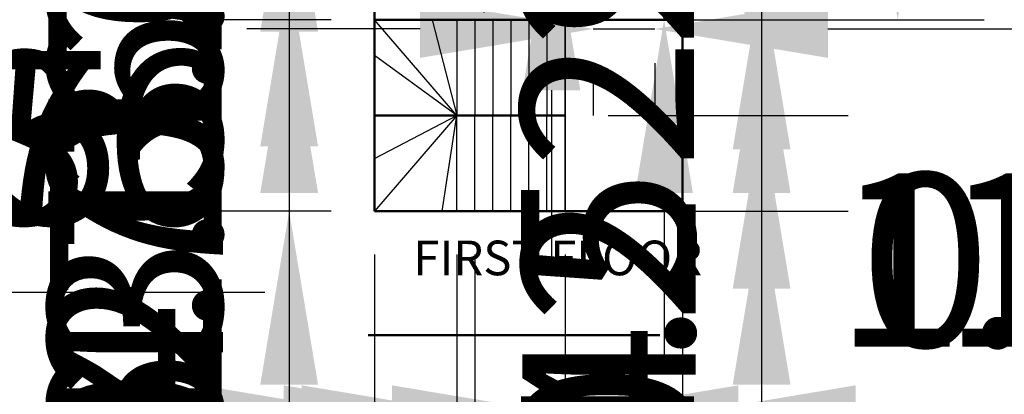
# Model space of a CAD drawing. Units: metres. Extents: x 782 to 1487, y 1262 to 7446.
# Tile 5 of 25: x 807.01 to 821.23, y 1287.66 to 1293.07. Entities that reach past the tile are written whole.
import ezdxf

# ---------------------------------------------------------------- set-up
doc = ezdxf.new("R2010")
doc.units = ezdxf.units.M
for name, color, linetype, lineweight in [('A-ANNO-DIMS', 2, 'Continuous', 18), ('A-ANNO-TEXT', 3, 'Continuous', 18), ('A-FLOR-STRS', 3, 'Continuous', 25), ('A-WALL', 7, 'Continuous', 50)]:
    doc.layers.add(name, color=color, linetype=linetype, lineweight=lineweight)
doc.styles.get("Standard").update_dxf_attribs({"font": 'arial.ttf'})
doc.dimstyles.new('ISO-25', dxfattribs={"dimtxt": 2.5, "dimasz": 2.5, "dimexe": 1.25, "dimexo": 0.625, "dimtad": 1, "dimtxsty": 'Standard', "dimcen": 2.5, "dimadec": 0, "dimazin": 0, "dimtfac": 1, "dimtmove": 0, "dimatfit": 3, "dimfxl": 1, "dimarcsym": 0})

# ---------------------------------------------------------------- blocks, each defined once
blk = doc.blocks.new('*D4')
at = {"layer": 'A-ANNO-DIMS', "color": 0, "lineweight": -2, "transparency": 16777216}
for p, q in [((817.205, 1307.327), (820.936, 1307.327)), ((819.686, 1304.827), (819.686, 1295.567)), ((817.205, 1293.067), (820.936, 1293.067))]:
    blk.add_line(p, q, dxfattribs=at)
at = {"layer": 'A-ANNO-DIMS', "color": 0, "transparency": 16777216}
for points in [[(819.269, 1304.827), (820.103, 1304.827), (819.686, 1307.327)], [(819.269, 1295.567), (820.103, 1295.567), (819.686, 1293.067)]]:
    blk.add_solid(points, dxfattribs=at)
at = {"layer": 'Defpoints', "color": 0, "transparency": 16777216}
for p in [(816.58, 1307.327), (816.58, 1293.067), (819.686, 1293.067)]:
    blk.add_point(p, dxfattribs=at)
at = {"layer": 'A-ANNO-DIMS', "color": 0, "transparency": 16777216, "insert": (817.558, 1300.197), "char_height": 2.5, "attachment_point": 5, "rotation": 90}
blk.add_mtext('14,26', dxfattribs=at)
blk = doc.blocks.new('*D22')
at = {"layer": 'A-ANNO-DIMS', "color": 0, "lineweight": -2, "transparency": 16777216}
for p, q in [((812.79, 1292.934), (810.29, 1292.934)), ((815.29, 1292.934), (816.179, 1292.934)), ((818.679, 1292.934), (848.834, 1292.934)), ((815.29, 1292.442), (815.29, 1291.684)), ((816.179, 1292.442), (816.179, 1291.684))]:
    blk.add_line(p, q, dxfattribs=at)
at = {"layer": 'A-ANNO-DIMS', "color": 0, "transparency": 16777216}
for points in [[(812.79, 1293.351), (812.79, 1292.517), (815.29, 1292.934)], [(818.679, 1293.351), (818.679, 1292.517), (816.179, 1292.934)]]:
    blk.add_solid(points, dxfattribs=at)
at = {"layer": 'Defpoints', "color": 0, "transparency": 16777216}
for p in [(815.29, 1293.067), (816.179, 1293.067), (816.179, 1292.934)]:
    blk.add_point(p, dxfattribs=at)
at = {"layer": 'A-ANNO-DIMS', "color": 0, "transparency": 16777216, "insert": (835.007, 1294.852), "char_height": 2.5, "attachment_point": 5}
blk.add_mtext('DOOR 0.89 TYP.', dxfattribs=at)
blk = doc.blocks.new('*D23')
at = {"layer": 'A-ANNO-DIMS', "color": 0, "lineweight": -2, "transparency": 16777216}
for p, q in [((816.313, 1296.414), (816.313, 1315.246)), ((816.313, 1293.067), (816.313, 1293.914)), ((816.804, 1293.914), (817.563, 1293.914)), ((816.804, 1293.067), (817.563, 1293.067)), ((816.313, 1290.567), (816.313, 1288.067))]:
    blk.add_line(p, q, dxfattribs=at)
at = {"layer": 'A-ANNO-DIMS', "color": 0, "transparency": 16777216}
for points in [[(815.896, 1296.414), (816.729, 1296.414), (816.313, 1293.914)], [(815.896, 1290.567), (816.729, 1290.567), (816.313, 1293.067)]]:
    blk.add_solid(points, dxfattribs=at)
at = {"layer": 'Defpoints', "color": 0, "transparency": 16777216}
for p in [(816.179, 1293.914), (816.313, 1293.914), (816.179, 1293.067)]:
    blk.add_point(p, dxfattribs=at)
at = {"layer": 'A-ANNO-DIMS', "color": 0, "transparency": 16777216, "insert": (814.411, 1307.08), "char_height": 2.5, "attachment_point": 5, "rotation": 90}
blk.add_mtext('0.85 TYP.', dxfattribs=at)
blk = doc.blocks.new('*D24')
at = {"layer": 'A-ANNO-DIMS', "color": 0, "lineweight": -2, "transparency": 16777216}
for p, q in [((811.209, 1294.423), (808.709, 1294.423)), ((813.709, 1294.423), (814.559, 1294.423)), ((817.059, 1294.423), (852.649, 1294.423)), ((813.709, 1293.926), (813.709, 1293.173)), ((814.559, 1293.926), (814.559, 1293.173))]:
    blk.add_line(p, q, dxfattribs=at)
at = {"layer": 'A-ANNO-DIMS', "color": 0, "transparency": 16777216}
for points in [[(811.209, 1294.84), (811.209, 1294.006), (813.709, 1294.423)], [(817.059, 1294.84), (817.059, 1294.006), (814.559, 1294.423)]]:
    blk.add_solid(points, dxfattribs=at)
at = {"layer": 'Defpoints', "color": 0, "transparency": 16777216}
for p in [(813.709, 1294.551), (814.559, 1294.551), (814.559, 1294.423)]:
    blk.add_point(p, dxfattribs=at)
at = {"layer": 'A-ANNO-DIMS', "color": 0, "transparency": 16777216, "insert": (836.104, 1296.342), "char_height": 2.5, "attachment_point": 5}
blk.add_mtext('DOOR D2 0.85 TYP.', dxfattribs=at)
blk = doc.blocks.new('*D25')
at = {"layer": 'A-ANNO-DIMS', "color": 0, "lineweight": -2, "transparency": 16777216}
for p, q in [((814.687, 1297.897), (814.687, 1316.729)), ((814.687, 1294.551), (814.687, 1295.397)), ((815.184, 1295.397), (815.937, 1295.397)), ((815.184, 1294.551), (815.937, 1294.551)), ((814.687, 1292.051), (814.687, 1289.551))]:
    blk.add_line(p, q, dxfattribs=at)
at = {"layer": 'A-ANNO-DIMS', "color": 0, "transparency": 16777216}
for points in [[(814.27, 1297.897), (815.103, 1297.897), (814.687, 1295.397)], [(814.27, 1292.051), (815.103, 1292.051), (814.687, 1294.551)]]:
    blk.add_solid(points, dxfattribs=at)
at = {"layer": 'Defpoints', "color": 0, "transparency": 16777216}
for p in [(814.559, 1295.397), (814.687, 1295.397), (814.559, 1294.551)]:
    blk.add_point(p, dxfattribs=at)
at = {"layer": 'A-ANNO-DIMS', "color": 0, "transparency": 16777216, "insert": (812.785, 1308.563), "char_height": 2.5, "attachment_point": 5, "rotation": 90}
blk.add_mtext('0.85 TYP.', dxfattribs=at)
blk = doc.blocks.new('*D48')
at = {"layer": 'A-ANNO-DIMS', "color": 0, "lineweight": -2, "transparency": 16777216}
for p, q in [((795.937, 1293.455), (795.937, 1287.89)), ((794.559, 1292.035), (794.559, 1287.89)), ((792.059, 1289.14), (789.559, 1289.14)), ((794.559, 1289.14), (795.937, 1289.14)), ((798.437, 1289.14), (808.45, 1289.14))]:
    blk.add_line(p, q, dxfattribs=at)
at = {"layer": 'A-ANNO-DIMS', "color": 0, "transparency": 16777216}
for points in [[(792.059, 1289.557), (792.059, 1288.724), (794.559, 1289.14)], [(798.437, 1289.557), (798.437, 1288.724), (795.937, 1289.14)]]:
    blk.add_solid(points, dxfattribs=at)
at = {"layer": 'Defpoints', "color": 0, "transparency": 16777216}
for p in [(795.937, 1294.08), (794.559, 1292.66), (795.937, 1289.14)]:
    blk.add_point(p, dxfattribs=at)
at = {"layer": 'A-ANNO-DIMS', "color": 0, "transparency": 16777216, "insert": (804.694, 1291.043), "char_height": 2.5, "attachment_point": 5}
blk.add_mtext('1.38', dxfattribs=at)
blk = doc.blocks.new('*D49')
at = {"layer": 'A-ANNO-DIMS', "color": 0, "lineweight": -2, "transparency": 16777216}
for p, q in [((795.937, 1292.035), (795.937, 1287.89)), ((796.288, 1292.035), (796.288, 1287.89)), ((793.437, 1289.14), (790.937, 1289.14)), ((795.937, 1289.14), (796.288, 1289.14)), ((798.788, 1289.14), (809.051, 1289.14))]:
    blk.add_line(p, q, dxfattribs=at)
at = {"layer": 'A-ANNO-DIMS', "color": 0, "transparency": 16777216}
for points in [[(793.437, 1289.557), (793.437, 1288.724), (795.937, 1289.14)], [(798.788, 1289.557), (798.788, 1288.724), (796.288, 1289.14)]]:
    blk.add_solid(points, dxfattribs=at)
at = {"layer": 'Defpoints', "color": 0, "transparency": 16777216}
for p in [(795.937, 1292.66), (796.288, 1292.66), (796.288, 1289.14)]:
    blk.add_point(p, dxfattribs=at)
at = {"layer": 'A-ANNO-DIMS', "color": 0, "transparency": 16777216, "insert": (805.169, 1291.043), "char_height": 2.5, "attachment_point": 5}
blk.add_mtext('0.35', dxfattribs=at)
blk = doc.blocks.new('*D50')
at = {"layer": 'A-ANNO-DIMS', "color": 0, "lineweight": -2, "transparency": 16777216}
for p, q in [((796.288, 1292.035), (796.288, 1287.89)), ((798.044, 1292.035), (798.044, 1287.89)), ((793.788, 1289.14), (791.288, 1289.14)), ((796.288, 1289.14), (798.044, 1289.14)), ((800.544, 1289.14), (810.551, 1289.14))]:
    blk.add_line(p, q, dxfattribs=at)
at = {"layer": 'A-ANNO-DIMS', "color": 0, "transparency": 16777216}
for points in [[(793.788, 1289.557), (793.788, 1288.724), (796.288, 1289.14)], [(800.544, 1289.557), (800.544, 1288.724), (798.044, 1289.14)]]:
    blk.add_solid(points, dxfattribs=at)
at = {"layer": 'Defpoints', "color": 0, "transparency": 16777216}
for p in [(796.288, 1292.66), (798.044, 1292.66), (798.044, 1289.14)]:
    blk.add_point(p, dxfattribs=at)
at = {"layer": 'A-ANNO-DIMS', "color": 0, "transparency": 16777216, "insert": (806.798, 1291.042), "char_height": 2.5, "attachment_point": 5}
blk.add_mtext('1.76', dxfattribs=at)
blk = doc.blocks.new('*D53')
at = {"layer": 'A-ANNO-DIMS', "color": 0, "lineweight": -2, "transparency": 16777216}
for p, q in [((810.9, 1309.827), (810.9, 1312.327)), ((811.505, 1307.327), (809.65, 1307.327)), ((810.9, 1307.327), (810.9, 1304.697)), ((811.735, 1304.697), (809.65, 1304.697)), ((810.9, 1302.197), (810.9, 1291.911))]:
    blk.add_line(p, q, dxfattribs=at)
at = {"layer": 'A-ANNO-DIMS', "color": 0, "transparency": 16777216}
for points in [[(810.483, 1309.827), (811.317, 1309.827), (810.9, 1307.327)], [(810.483, 1302.197), (811.317, 1302.197), (810.9, 1304.697)]]:
    blk.add_solid(points, dxfattribs=at)
at = {"layer": 'Defpoints', "color": 0, "transparency": 16777216}
for p in [(812.13, 1307.327), (810.9, 1304.697), (812.36, 1304.697)]:
    blk.add_point(p, dxfattribs=at)
at = {"layer": 'A-ANNO-DIMS', "color": 0, "transparency": 16777216, "insert": (808.998, 1295.804), "char_height": 2.5, "attachment_point": 5, "rotation": 90}
blk.add_mtext('2.63', dxfattribs=at)
blk = doc.blocks.new('*D54')
at = {"layer": 'A-ANNO-DIMS', "color": 0, "lineweight": -2, "transparency": 16777216}
for p, q in [((810.9, 1307.197), (810.9, 1309.697)), ((811.735, 1304.697), (809.65, 1304.697)), ((810.9, 1304.697), (810.9, 1302.822)), ((811.503, 1302.822), (809.65, 1302.822)), ((810.9, 1300.322), (810.9, 1290.308))]:
    blk.add_line(p, q, dxfattribs=at)
at = {"layer": 'A-ANNO-DIMS', "color": 0, "transparency": 16777216}
for points in [[(810.483, 1307.197), (811.317, 1307.197), (810.9, 1304.697)], [(810.483, 1300.322), (811.317, 1300.322), (810.9, 1302.822)]]:
    blk.add_solid(points, dxfattribs=at)
at = {"layer": 'Defpoints', "color": 0, "transparency": 16777216}
for p in [(812.36, 1304.697), (810.9, 1302.822), (812.128, 1302.822)]:
    blk.add_point(p, dxfattribs=at)
at = {"layer": 'A-ANNO-DIMS', "color": 0, "transparency": 16777216, "insert": (808.999, 1294.065), "char_height": 2.5, "attachment_point": 5, "rotation": 90}
blk.add_mtext('1.88', dxfattribs=at)
blk = doc.blocks.new('*D55')
at = {"layer": 'A-ANNO-DIMS', "color": 0, "lineweight": -2, "transparency": 16777216}
for p, q in [((810.9, 1305.322), (810.9, 1307.822)), ((811.503, 1302.822), (809.65, 1302.822)), ((810.9, 1302.822), (810.9, 1302.177)), ((811.735, 1302.177), (809.65, 1302.177)), ((810.9, 1299.677), (810.9, 1289.444))]:
    blk.add_line(p, q, dxfattribs=at)
at = {"layer": 'A-ANNO-DIMS', "color": 0, "transparency": 16777216}
for points in [[(810.483, 1305.322), (811.317, 1305.322), (810.9, 1302.822)], [(810.483, 1299.677), (811.317, 1299.677), (810.9, 1302.177)]]:
    blk.add_solid(points, dxfattribs=at)
at = {"layer": 'Defpoints', "color": 0, "transparency": 16777216}
for p in [(812.128, 1302.822), (810.9, 1302.177), (812.36, 1302.177)]:
    blk.add_point(p, dxfattribs=at)
at = {"layer": 'A-ANNO-DIMS', "color": 0, "transparency": 16777216, "insert": (808.999, 1293.311), "char_height": 2.5, "attachment_point": 5, "rotation": 90}
blk.add_mtext('0.64', dxfattribs=at)
blk = doc.blocks.new('*D56')
at = {"layer": 'A-ANNO-DIMS', "color": 0, "lineweight": -2, "transparency": 16777216}
for p, q in [((810.9, 1304.677), (810.9, 1307.177)), ((811.735, 1302.177), (809.65, 1302.177)), ((810.9, 1302.177), (810.9, 1299.809)), ((811.505, 1299.809), (809.65, 1299.809)), ((810.9, 1297.309), (810.9, 1287.022))]:
    blk.add_line(p, q, dxfattribs=at)
at = {"layer": 'A-ANNO-DIMS', "color": 0, "transparency": 16777216}
for points in [[(810.483, 1304.677), (811.317, 1304.677), (810.9, 1302.177)], [(810.483, 1297.309), (811.317, 1297.309), (810.9, 1299.809)]]:
    blk.add_solid(points, dxfattribs=at)
at = {"layer": 'Defpoints', "color": 0, "transparency": 16777216}
for p in [(812.36, 1302.177), (810.9, 1299.809), (812.13, 1299.809)]:
    blk.add_point(p, dxfattribs=at)
at = {"layer": 'A-ANNO-DIMS', "color": 0, "transparency": 16777216, "insert": (808.998, 1290.916), "char_height": 2.5, "attachment_point": 5, "rotation": 90}
blk.add_mtext('2.37', dxfattribs=at)
blk = doc.blocks.new('*D57')
at = {"layer": 'A-ANNO-DIMS', "color": 0, "lineweight": -2, "transparency": 16777216}
for p, q in [((810.9, 1302.309), (810.9, 1304.809)), ((811.505, 1299.809), (809.65, 1299.809)), ((810.9, 1299.809), (810.9, 1298.647)), ((811.735, 1298.647), (809.65, 1298.647)), ((810.9, 1296.147), (810.9, 1286.141))]:
    blk.add_line(p, q, dxfattribs=at)
at = {"layer": 'A-ANNO-DIMS', "color": 0, "transparency": 16777216}
for points in [[(810.483, 1302.309), (811.317, 1302.309), (810.9, 1299.809)], [(810.483, 1296.147), (811.317, 1296.147), (810.9, 1298.647)]]:
    blk.add_solid(points, dxfattribs=at)
at = {"layer": 'Defpoints', "color": 0, "transparency": 16777216}
for p in [(812.13, 1299.809), (810.9, 1298.647), (812.36, 1298.647)]:
    blk.add_point(p, dxfattribs=at)
at = {"layer": 'A-ANNO-DIMS', "color": 0, "transparency": 16777216, "insert": (808.999, 1289.894), "char_height": 2.5, "attachment_point": 5, "rotation": 90}
blk.add_mtext('1.16', dxfattribs=at)
blk = doc.blocks.new('*D58')
at = {"layer": 'A-ANNO-DIMS', "color": 0, "lineweight": -2, "transparency": 16777216}
for p, q in [((810.9, 1301.147), (810.9, 1303.647)), ((811.735, 1298.647), (809.65, 1298.647)), ((810.9, 1298.647), (810.9, 1296.5)), ((811.507, 1296.5), (809.65, 1296.5)), ((810.9, 1294), (810.9, 1281.772))]:
    blk.add_line(p, q, dxfattribs=at)
at = {"layer": 'A-ANNO-DIMS', "color": 0, "transparency": 16777216}
for points in [[(810.483, 1301.147), (811.317, 1301.147), (810.9, 1298.647)], [(810.483, 1294), (811.317, 1294), (810.9, 1296.5)]]:
    blk.add_solid(points, dxfattribs=at)
at = {"layer": 'Defpoints', "color": 0, "transparency": 16777216}
for p in [(812.36, 1298.647), (810.9, 1296.5), (812.132, 1296.5)]:
    blk.add_point(p, dxfattribs=at)
at = {"layer": 'A-ANNO-DIMS', "color": 0, "transparency": 16777216, "insert": (809.02, 1286.636), "char_height": 2.5, "attachment_point": 5, "rotation": 90}
blk.add_mtext('2.147', dxfattribs=at)
blk = doc.blocks.new('*D59')
at = {"layer": 'A-ANNO-DIMS', "color": 0, "lineweight": -2, "transparency": 16777216}
for p, q in [((810.9, 1299), (810.9, 1301.5)), ((811.507, 1296.5), (809.65, 1296.5)), ((810.9, 1296.5), (810.9, 1295.397)), ((811.735, 1295.397), (809.65, 1295.397)), ((810.9, 1292.897), (810.9, 1280.947))]:
    blk.add_line(p, q, dxfattribs=at)
at = {"layer": 'A-ANNO-DIMS', "color": 0, "transparency": 16777216}
for points in [[(810.483, 1299), (811.317, 1299), (810.9, 1296.5)], [(810.483, 1292.897), (811.317, 1292.897), (810.9, 1295.397)]]:
    blk.add_solid(points, dxfattribs=at)
at = {"layer": 'Defpoints', "color": 0, "transparency": 16777216}
for p in [(812.132, 1296.5), (810.9, 1295.397), (812.36, 1295.397)]:
    blk.add_point(p, dxfattribs=at)
at = {"layer": 'A-ANNO-DIMS', "color": 0, "transparency": 16777216, "insert": (808.998, 1285.672), "char_height": 2.5, "attachment_point": 5, "rotation": 90}
blk.add_mtext('1.103', dxfattribs=at)
blk = doc.blocks.new('*D60')
at = {"layer": 'A-ANNO-DIMS', "color": 0, "lineweight": -2, "transparency": 16777216}
for p, q in [((810.9, 1297.897), (810.9, 1300.397)), ((811.735, 1295.397), (809.65, 1295.397)), ((810.9, 1295.397), (810.9, 1293.74)), ((811.505, 1293.74), (809.65, 1293.74)), ((810.9, 1291.24), (810.9, 1281.233))]:
    blk.add_line(p, q, dxfattribs=at)
at = {"layer": 'A-ANNO-DIMS', "color": 0, "transparency": 16777216}
for points in [[(810.483, 1297.897), (811.317, 1297.897), (810.9, 1295.397)], [(810.483, 1291.24), (811.317, 1291.24), (810.9, 1293.74)]]:
    blk.add_solid(points, dxfattribs=at)
at = {"layer": 'Defpoints', "color": 0, "transparency": 16777216}
for p in [(812.36, 1295.397), (810.9, 1293.74), (812.13, 1293.74)]:
    blk.add_point(p, dxfattribs=at)
at = {"layer": 'A-ANNO-DIMS', "color": 0, "transparency": 16777216, "insert": (808.999, 1284.987), "char_height": 2.5, "attachment_point": 5, "rotation": 90}
blk.add_mtext('1.66', dxfattribs=at)
blk = doc.blocks.new('*D61')
at = {"layer": 'A-ANNO-DIMS', "color": 0, "lineweight": -2, "transparency": 16777216}
for p, q in [((810.9, 1296.24), (810.9, 1298.74)), ((811.505, 1293.74), (809.65, 1293.74)), ((810.9, 1293.74), (810.9, 1293.067)), ((811.505, 1293.067), (809.65, 1293.067)), ((810.9, 1290.567), (810.9, 1280.324))]:
    blk.add_line(p, q, dxfattribs=at)
at = {"layer": 'A-ANNO-DIMS', "color": 0, "transparency": 16777216}
for points in [[(810.483, 1296.24), (811.317, 1296.24), (810.9, 1293.74)], [(810.483, 1290.567), (811.317, 1290.567), (810.9, 1293.067)]]:
    blk.add_solid(points, dxfattribs=at)
at = {"layer": 'Defpoints', "color": 0, "transparency": 16777216}
for p in [(812.13, 1293.74), (810.9, 1293.067), (812.13, 1293.067)]:
    blk.add_point(p, dxfattribs=at)
at = {"layer": 'A-ANNO-DIMS', "color": 0, "transparency": 16777216, "insert": (808.999, 1284.195), "char_height": 2.5, "attachment_point": 5, "rotation": 90}
blk.add_mtext('0.67', dxfattribs=at)
blk = doc.blocks.new('*D62')
at = {"layer": 'A-ANNO-DIMS', "color": 0, "lineweight": -2, "transparency": 16777216}
for p, q in [((810.9, 1295.567), (810.9, 1298.067)), ((811.505, 1293.067), (809.65, 1293.067)), ((810.9, 1293.067), (810.9, 1290.305)), ((811.505, 1290.305), (809.65, 1290.305)), ((810.9, 1287.805), (810.9, 1275.602))]:
    blk.add_line(p, q, dxfattribs=at)
at = {"layer": 'A-ANNO-DIMS', "color": 0, "transparency": 16777216}
for points in [[(810.483, 1295.567), (811.317, 1295.567), (810.9, 1293.067)], [(810.483, 1287.805), (811.317, 1287.805), (810.9, 1290.305)]]:
    blk.add_solid(points, dxfattribs=at)
at = {"layer": 'Defpoints', "color": 0, "transparency": 16777216}
for p in [(812.13, 1293.067), (810.9, 1290.305), (812.13, 1290.305)]:
    blk.add_point(p, dxfattribs=at)
at = {"layer": 'A-ANNO-DIMS', "color": 0, "transparency": 16777216, "insert": (808.999, 1280.454), "char_height": 2.5, "attachment_point": 5, "rotation": 90}
blk.add_mtext('2.762', dxfattribs=at)
blk = doc.blocks.new('*D63')
at = {"layer": 'A-ANNO-DIMS', "color": 0, "lineweight": -2, "transparency": 16777216}
for p, q in [((817.721, 1309.827), (817.721, 1312.327)), ((817.205, 1307.327), (818.971, 1307.327)), ((817.721, 1307.327), (817.721, 1304.867)), ((817.205, 1304.867), (818.971, 1304.867)), ((817.721, 1302.367), (817.721, 1292.082))]:
    blk.add_line(p, q, dxfattribs=at)
at = {"layer": 'A-ANNO-DIMS', "color": 0, "transparency": 16777216}
for points in [[(817.304, 1309.827), (818.138, 1309.827), (817.721, 1307.327)], [(817.304, 1302.367), (818.138, 1302.367), (817.721, 1304.867)]]:
    blk.add_solid(points, dxfattribs=at)
at = {"layer": 'Defpoints', "color": 0, "transparency": 16777216}
for p in [(816.58, 1307.327), (816.58, 1304.867), (817.721, 1304.867)]:
    blk.add_point(p, dxfattribs=at)
at = {"layer": 'A-ANNO-DIMS', "color": 0, "transparency": 16777216, "insert": (815.82, 1295.974), "char_height": 2.5, "attachment_point": 5, "rotation": 90}
blk.add_mtext('2.46', dxfattribs=at)
blk = doc.blocks.new('*D64')
at = {"layer": 'A-ANNO-DIMS', "color": 0, "lineweight": -2, "transparency": 16777216}
for p, q in [((817.721, 1307.367), (817.721, 1309.867)), ((817.205, 1304.867), (818.971, 1304.867)), ((817.721, 1304.867), (817.721, 1300.338)), ((817.206, 1300.338), (818.971, 1300.338)), ((817.721, 1297.838), (817.721, 1285.546))]:
    blk.add_line(p, q, dxfattribs=at)
at = {"layer": 'A-ANNO-DIMS', "color": 0, "transparency": 16777216}
for points in [[(817.304, 1307.367), (818.138, 1307.367), (817.721, 1304.867)], [(817.304, 1297.838), (818.138, 1297.838), (817.721, 1300.338)]]:
    blk.add_solid(points, dxfattribs=at)
at = {"layer": 'Defpoints', "color": 0, "transparency": 16777216}
for p in [(816.58, 1304.867), (816.581, 1300.338), (817.721, 1300.338)]:
    blk.add_point(p, dxfattribs=at)
at = {"layer": 'A-ANNO-DIMS', "color": 0, "transparency": 16777216, "insert": (815.82, 1290.442), "char_height": 2.5, "attachment_point": 5, "rotation": 90}
blk.add_mtext('4.529', dxfattribs=at)
blk = doc.blocks.new('*D65')
at = {"layer": 'A-ANNO-DIMS', "color": 0, "lineweight": -2, "transparency": 16777216}
for p, q in [((817.721, 1302.838), (817.721, 1305.338)), ((817.206, 1300.338), (818.971, 1300.338)), ((817.721, 1300.338), (817.721, 1296.196)), ((817.205, 1296.196), (818.971, 1296.196)), ((817.721, 1293.696), (817.721, 1281.435))]:
    blk.add_line(p, q, dxfattribs=at)
at = {"layer": 'A-ANNO-DIMS', "color": 0, "transparency": 16777216}
for points in [[(817.304, 1302.838), (818.138, 1302.838), (817.721, 1300.338)], [(817.304, 1293.696), (818.138, 1293.696), (817.721, 1296.196)]]:
    blk.add_solid(points, dxfattribs=at)
at = {"layer": 'Defpoints', "color": 0, "transparency": 16777216}
for p in [(816.581, 1300.338), (816.58, 1296.196), (817.721, 1296.196)]:
    blk.add_point(p, dxfattribs=at)
at = {"layer": 'A-ANNO-DIMS', "color": 0, "transparency": 16777216, "insert": (815.841, 1286.315), "char_height": 2.5, "attachment_point": 5, "rotation": 90}
blk.add_mtext('4.142', dxfattribs=at)
blk = doc.blocks.new('*D66')
at = {"layer": 'A-ANNO-DIMS', "color": 0, "lineweight": -2, "transparency": 16777216}
for p, q in [((817.721, 1298.696), (817.721, 1301.196)), ((817.205, 1296.196), (818.971, 1296.196)), ((817.721, 1296.196), (817.721, 1293.699)), ((817.205, 1293.699), (818.971, 1293.699)), ((817.721, 1291.199), (817.721, 1280.921))]:
    blk.add_line(p, q, dxfattribs=at)
at = {"layer": 'A-ANNO-DIMS', "color": 0, "transparency": 16777216}
for points in [[(817.304, 1298.696), (818.138, 1298.696), (817.721, 1296.196)], [(817.304, 1291.199), (818.138, 1291.199), (817.721, 1293.699)]]:
    blk.add_solid(points, dxfattribs=at)
at = {"layer": 'Defpoints', "color": 0, "transparency": 16777216}
for p in [(816.58, 1296.196), (816.58, 1293.699), (817.721, 1293.699)]:
    blk.add_point(p, dxfattribs=at)
at = {"layer": 'A-ANNO-DIMS', "color": 0, "transparency": 16777216, "insert": (815.82, 1284.81), "char_height": 2.5, "attachment_point": 5, "rotation": 90}
blk.add_mtext('2.50', dxfattribs=at)
blk = doc.blocks.new('*D67')
at = {"layer": 'A-ANNO-DIMS', "color": 0, "lineweight": -2, "transparency": 16777216}
for p, q in [((817.721, 1296.199), (817.721, 1298.699)), ((817.205, 1293.699), (818.971, 1293.699)), ((817.721, 1293.699), (817.721, 1293.067)), ((817.205, 1293.067), (818.971, 1293.067)), ((817.721, 1290.567), (817.721, 1278.407))]:
    blk.add_line(p, q, dxfattribs=at)
at = {"layer": 'A-ANNO-DIMS', "color": 0, "transparency": 16777216}
for points in [[(817.304, 1296.199), (818.138, 1296.199), (817.721, 1293.699)], [(817.304, 1290.567), (818.138, 1290.567), (817.721, 1293.067)]]:
    blk.add_solid(points, dxfattribs=at)
at = {"layer": 'Defpoints', "color": 0, "transparency": 16777216}
for p in [(816.58, 1293.699), (816.58, 1293.067), (817.721, 1293.067)]:
    blk.add_point(p, dxfattribs=at)
at = {"layer": 'A-ANNO-DIMS', "color": 0, "transparency": 16777216, "insert": (815.819, 1283.237), "char_height": 2.5, "attachment_point": 5, "rotation": 90}
blk.add_mtext('0.632', dxfattribs=at)
blk = doc.blocks.new('*D68')
at = {"layer": 'A-ANNO-DIMS', "color": 0, "lineweight": -2, "transparency": 16777216}
for p, q in [((817.721, 1295.567), (817.721, 1298.067)), ((815.508, 1293.067), (818.971, 1293.067)), ((817.721, 1293.067), (817.721, 1291.686)), ((815.508, 1291.686), (818.971, 1291.686)), ((817.721, 1289.186), (817.721, 1277.718))]:
    blk.add_line(p, q, dxfattribs=at)
at = {"layer": 'A-ANNO-DIMS', "color": 0, "transparency": 16777216}
for points in [[(817.304, 1295.567), (818.138, 1295.567), (817.721, 1293.067)], [(817.304, 1289.186), (818.138, 1289.186), (817.721, 1291.686)]]:
    blk.add_solid(points, dxfattribs=at)
at = {"layer": 'Defpoints', "color": 0, "transparency": 16777216}
for p in [(814.883, 1293.067), (814.883, 1291.686), (817.721, 1291.686)]:
    blk.add_point(p, dxfattribs=at)
at = {"layer": 'A-ANNO-DIMS', "color": 0, "transparency": 16777216, "insert": (815.819, 1282.202), "char_height": 2.5, "attachment_point": 5, "rotation": 90}
blk.add_mtext('1.381', dxfattribs=at)
blk = doc.blocks.new('*D69')
at = {"layer": 'A-ANNO-DIMS', "color": 0, "lineweight": -2, "transparency": 16777216}
for p, q in [((817.721, 1294.186), (817.721, 1296.686)), ((815.508, 1291.686), (818.971, 1291.686)), ((817.721, 1291.686), (817.721, 1290.305)), ((815.508, 1290.305), (818.971, 1290.305)), ((817.721, 1287.805), (817.721, 1276.337))]:
    blk.add_line(p, q, dxfattribs=at)
at = {"layer": 'A-ANNO-DIMS', "color": 0, "transparency": 16777216}
for points in [[(817.304, 1294.186), (818.138, 1294.186), (817.721, 1291.686)], [(817.304, 1287.805), (818.138, 1287.805), (817.721, 1290.305)]]:
    blk.add_solid(points, dxfattribs=at)
at = {"layer": 'Defpoints', "color": 0, "transparency": 16777216}
for p in [(814.883, 1291.686), (814.883, 1290.305), (817.721, 1290.305)]:
    blk.add_point(p, dxfattribs=at)
at = {"layer": 'A-ANNO-DIMS', "color": 0, "transparency": 16777216, "insert": (815.819, 1280.821), "char_height": 2.5, "attachment_point": 5, "rotation": 90}
blk.add_mtext('1.381', dxfattribs=at)
blk = doc.blocks.new('*D73')
at = {"layer": 'A-ANNO-DIMS', "color": 0, "lineweight": -2, "transparency": 16777216}
for p, q in [((812.13, 1289.68), (812.13, 1286.127)), ((813.319, 1289.68), (813.319, 1286.127)), ((809.63, 1287.377), (807.13, 1287.377)), ((812.13, 1287.377), (813.319, 1287.377)), ((815.819, 1287.377), (825.832, 1287.377))]:
    blk.add_line(p, q, dxfattribs=at)
at = {"layer": 'A-ANNO-DIMS', "color": 0, "transparency": 16777216}
for points in [[(809.63, 1287.794), (809.63, 1286.96), (812.13, 1287.377)], [(815.819, 1287.794), (815.819, 1286.96), (813.319, 1287.377)]]:
    blk.add_solid(points, dxfattribs=at)
at = {"layer": 'Defpoints', "color": 0, "transparency": 16777216}
for p in [(812.13, 1290.305), (813.319, 1290.305), (813.319, 1287.377)]:
    blk.add_point(p, dxfattribs=at)
at = {"layer": 'A-ANNO-DIMS', "color": 0, "transparency": 16777216, "insert": (822.076, 1289.278), "char_height": 2.5, "attachment_point": 5}
blk.add_mtext('1.19', dxfattribs=at)
blk = doc.blocks.new('*D74')
at = {"layer": 'A-ANNO-DIMS', "color": 0, "lineweight": -2, "transparency": 16777216}
for p, q in [((813.319, 1289.68), (813.319, 1286.127)), ((813.58, 1289.68), (813.58, 1286.127)), ((810.819, 1287.377), (808.319, 1287.377)), ((813.319, 1287.377), (813.58, 1287.377)), ((816.08, 1287.377), (826.322, 1287.377))]:
    blk.add_line(p, q, dxfattribs=at)
at = {"layer": 'A-ANNO-DIMS', "color": 0, "transparency": 16777216}
for points in [[(810.819, 1287.794), (810.819, 1286.96), (813.319, 1287.377)], [(816.08, 1287.794), (816.08, 1286.96), (813.58, 1287.377)]]:
    blk.add_solid(points, dxfattribs=at)
at = {"layer": 'Defpoints', "color": 0, "transparency": 16777216}
for p in [(813.319, 1290.305), (813.58, 1290.305), (813.58, 1287.377)]:
    blk.add_point(p, dxfattribs=at)
at = {"layer": 'A-ANNO-DIMS', "color": 0, "transparency": 16777216, "insert": (822.451, 1289.278), "char_height": 2.5, "attachment_point": 5}
blk.add_mtext('0.26', dxfattribs=at)
blk = doc.blocks.new('*D75')
at = {"layer": 'A-ANNO-DIMS', "color": 0, "lineweight": -2, "transparency": 16777216}
for p, q in [((813.58, 1289.68), (813.58, 1286.127)), ((814.883, 1289.68), (814.883, 1286.127)), ((811.08, 1287.377), (808.58, 1287.377)), ((813.58, 1287.377), (814.883, 1287.377)), ((817.383, 1287.377), (827.383, 1287.377))]:
    blk.add_line(p, q, dxfattribs=at)
at = {"layer": 'A-ANNO-DIMS', "color": 0, "transparency": 16777216}
for points in [[(811.08, 1287.794), (811.08, 1286.96), (813.58, 1287.377)], [(817.383, 1287.794), (817.383, 1286.96), (814.883, 1287.377)]]:
    blk.add_solid(points, dxfattribs=at)
at = {"layer": 'Defpoints', "color": 0, "transparency": 16777216}
for p in [(813.58, 1290.305), (814.883, 1290.305), (814.883, 1287.377)]:
    blk.add_point(p, dxfattribs=at)
at = {"layer": 'A-ANNO-DIMS', "color": 0, "transparency": 16777216, "insert": (823.633, 1289.279), "char_height": 2.5, "attachment_point": 5}
blk.add_mtext('1.30', dxfattribs=at)
blk = doc.blocks.new('*D76')
at = {"layer": 'A-ANNO-DIMS', "color": 0, "lineweight": -2, "transparency": 16777216}
for p, q in [((814.883, 1289.68), (814.883, 1286.127)), ((816.58, 1289.68), (816.58, 1286.127)), ((812.383, 1287.377), (809.883, 1287.377)), ((814.883, 1287.377), (816.58, 1287.377)), ((819.08, 1287.377), (831.031, 1287.377))]:
    blk.add_line(p, q, dxfattribs=at)
at = {"layer": 'A-ANNO-DIMS', "color": 0, "transparency": 16777216}
for points in [[(812.383, 1287.794), (812.383, 1286.96), (814.883, 1287.377)], [(819.08, 1287.794), (819.08, 1286.96), (816.58, 1287.377)]]:
    blk.add_solid(points, dxfattribs=at)
at = {"layer": 'Defpoints', "color": 0, "transparency": 16777216}
for p in [(814.883, 1290.305), (816.58, 1290.305), (816.58, 1287.377)]:
    blk.add_point(p, dxfattribs=at)
at = {"layer": 'A-ANNO-DIMS', "color": 0, "transparency": 16777216, "insert": (826.305, 1289.278), "char_height": 2.5, "attachment_point": 5}
blk.add_mtext('1.697', dxfattribs=at)

msp = doc.modelspace()

# ---------------------------------------------------------------- linework, layer by layer
at = {"layer": 'A-FLOR-STRS'}
for p, q in [((813.3188, 1291.6863), (812.13, 1293.0674)), ((813.3188, 1293.0674), (812.965, 1293.0674)), ((812.965, 1293.0674), (813.3188, 1291.6863)), ((813.3188, 1293.0674), (813.3188, 1291.6863)), ((813.5796, 1293.0674), (813.5796, 1291.6863)), ((813.8403, 1293.0674), (813.8403, 1291.6863)), ((814.101, 1293.0674), (814.101, 1291.6863)), ((814.3617, 1293.0674), (814.3617, 1291.6863)), ((814.6224, 1293.0674), (814.6224, 1291.6863)), ((814.8832, 1290.3053), (814.8832, 1293.0674)), ((814.8832, 1293.0674), (814.8832, 1290.3053)), ((814.8832, 1293.0674), (814.8832, 1291.6863)), ((813.3188, 1291.6863), (812.13, 1292.5526)), ((813.3188, 1291.6863), (812.13, 1290.3053)), ((813.3188, 1291.6863), (812.13, 1291.6863)), ((812.13, 1291.0666), (813.3188, 1291.6863)), ((813.1108, 1290.3053), (813.3188, 1291.6863)), ((813.3188, 1290.3053), (813.3188, 1291.6863)), ((813.5796, 1290.3053), (813.5796, 1291.6863)), ((813.8403, 1290.3053), (813.8403, 1291.6863)), ((814.101, 1290.3053), (814.101, 1291.6863)), ((814.3617, 1290.3053), (814.3617, 1291.6863)), ((814.6224, 1290.3053), (814.6224, 1291.6863)), ((814.8832, 1290.3053), (814.8832, 1291.6863))]:
    msp.add_line(p, q, dxfattribs=at)
at = {"layer": 'A-WALL'}
for p, q in [((816.58, 1303.3374), (816.58, 1293.0674)), ((812.13, 1295.3974), (812.13, 1293.0674)), ((812.13, 1293.0674), (814.84, 1293.0674)), ((812.13, 1293.0674), (812.13, 1290.3053)), ((816.58, 1293.0674), (812.13, 1293.0674)), ((814.84, 1293.0674), (815.3293, 1293.0674)), ((816.1414, 1293.0674), (816.58, 1293.0674)), ((816.23, 1293.0674), (816.1792, 1293.0674)), ((816.58, 1290.3053), (816.58, 1293.0674)), ((814.8832, 1291.6863), (812.13, 1291.6863)), ((814.8832, 1291.6863), (812.13, 1291.6863)), ((812.13, 1291.6863), (812.13, 1291.0666)), ((812.13, 1290.3053), (816.58, 1290.3053)), ((812.13, 1290.3053), (813.1108, 1290.3053)), ((812.04, 1288.517), (816.2494, 1288.517))]:
    msp.add_line(p, q, dxfattribs=at)

# ---------------------------------------------------------------- texts
at = {"layer": 'A-ANNO-TEXT', "insert": (812.6929, 1289.8815), "char_height": 0.5, "attachment_point": 1}
msp.add_mtext_dynamic_manual_height_columns('FIRST FLOOR', width=4.459798, gutter_width=12.5, heights=[0], dxfattribs=at)

# ---------------------------------------------------------------- dimensions: what is measured, and where the dimension line sits
at = {"layer": 'A-ANNO-DIMS'}
for base, p1, p2, picture, middle in [((814.6868, 1295.3974), (814.5592, 1294.5507), (814.5592, 1295.3974), '*D25', (812.7854, 1308.5633)), ((816.3126, 1293.9141), (816.1792, 1293.0674), (816.1792, 1293.9141), '*D23', (814.4112, 1307.08))]:
    dim = msp.add_linear_dim(base=base, p1=p1, p2=p2, angle=90, text='<> TYP.', dimstyle='ISO-25', override={"dimdec": 2, "dimlfac": 1, "dimrnd": 0, "dimzin": 0, "dimdsep": 46, "dimlunit": 2}, dxfattribs=at)
    dim.commit()
    dim.dimension.update_dxf_attribs({"geometry": picture, "text_midpoint": middle})
for base, p1, p2, override, picture, middle in [((810.9, 1304.6974), (812.13, 1307.3274), (812.36, 1304.6974), {"dimdec": 2, "dimlfac": 1, "dimrnd": 0, "dimzin": 0, "dimdsep": 46, "dimlunit": 2}, '*D53', (808.9978, 1295.8042)), ((817.7211, 1304.8669), (816.58, 1307.3274), (816.5802, 1304.8669), {"dimdec": 2, "dimlfac": 1, "dimrnd": 0, "dimzin": 0, "dimdsep": 46, "dimlunit": 2}, '*D63', (815.8196, 1295.9745)), ((817.7211, 1300.3378), (816.5802, 1304.8669), (816.5811, 1300.3378), {"dimdec": 3, "dimlfac": 1, "dimrnd": 0, "dimzin": 0, "dimdsep": 46, "dimlunit": 2}, '*D64', (815.8196, 1290.4419)), ((810.9, 1302.8221), (812.36, 1304.6974), (812.1285, 1302.8221), {"dimdec": 2, "dimlfac": 1, "dimrnd": 0, "dimzin": 0, "dimdsep": 46, "dimlunit": 2}, '*D54', (808.9986, 1294.0652)), ((810.9, 1302.1774), (812.1285, 1302.8221), (812.36, 1302.1774), {"dimdec": 2, "dimlfac": 1, "dimrnd": 0, "dimzin": 0, "dimdsep": 46, "dimlunit": 2}, '*D55', (808.9986, 1293.3106)), ((819.6859, 1293.0674), (816.58, 1307.3274), (816.58, 1293.0674), {"dimclrd": 0, "dimclre": 0, "dimclrt": 0}, '*D4', (817.5585, 1300.1974)), ((810.9, 1299.8088), (812.36, 1302.1774), (812.1301, 1299.8088), {"dimdec": 2, "dimlfac": 1, "dimrnd": 0, "dimzin": 0, "dimdsep": 46, "dimlunit": 2}, '*D56', (808.9978, 1290.9156)), ((817.7211, 1296.196), (816.5811, 1300.3378), (816.58, 1296.196), {"dimdec": 3, "dimlfac": 1, "dimrnd": 0, "dimzin": 0, "dimdsep": 46, "dimlunit": 2}, '*D65', (815.8409, 1286.3153)), ((810.9, 1298.6474), (812.1301, 1299.8088), (812.36, 1298.6474), {"dimdec": 2, "dimlfac": 1, "dimrnd": 0, "dimzin": 0, "dimdsep": 46, "dimlunit": 2}, '*D57', (808.9986, 1289.894)), ((810.9, 1296.5004), (812.36, 1298.6474), (812.1317, 1296.5004), {"dimdec": 3, "dimlfac": 1, "dimrnd": 0, "dimzin": 0, "dimdsep": 46, "dimlunit": 2}, '*D58', (809.0199, 1286.636)), ((810.9, 1295.3974), (812.1317, 1296.5004), (812.36, 1295.3974), {"dimdec": 3, "dimlfac": 1, "dimrnd": 0, "dimzin": 0, "dimdsep": 46, "dimlunit": 2}, '*D59', (808.9978, 1285.672)), ((817.7211, 1293.6994), (816.58, 1296.196), (816.58, 1293.6994), {"dimdec": 2, "dimlfac": 1, "dimrnd": 0, "dimzin": 0, "dimdsep": 46, "dimlunit": 2}, '*D66', (815.8196, 1284.8104)), ((810.9, 1293.7402), (812.36, 1295.3974), (812.1297, 1293.7402), {"dimdec": 2, "dimlfac": 1, "dimrnd": 0, "dimzin": 0, "dimdsep": 46, "dimlunit": 2}, '*D60', (808.9986, 1284.9868)), ((810.9, 1293.0674), (812.1297, 1293.7402), (812.13, 1293.0674), {"dimdec": 2, "dimlfac": 1, "dimrnd": 0, "dimzin": 0, "dimdsep": 46, "dimlunit": 2}, '*D61', (808.9986, 1284.1955)), ((817.7211, 1293.0674), (816.58, 1293.6994), (816.58, 1293.0674), {"dimdec": 3, "dimlfac": 1, "dimrnd": 0, "dimzin": 0, "dimdsep": 46, "dimlunit": 2}, '*D67', (815.8188, 1283.2371)), ((810.9, 1290.3053), (812.13, 1293.0674), (812.13, 1290.3053), {"dimdec": 3, "dimlfac": 1, "dimrnd": 0, "dimzin": 0, "dimdsep": 46, "dimlunit": 2}, '*D62', (808.9986, 1280.4536)), ((817.7211, 1291.6863), (814.8832, 1293.0674), (814.8832, 1291.6863), {"dimdec": 3, "dimlfac": 1, "dimrnd": 0, "dimzin": 0, "dimdsep": 46, "dimlunit": 2}, '*D68', (815.8188, 1282.2022)), ((817.7211, 1290.3053), (814.8832, 1291.6863), (814.8832, 1290.3053), {"dimdec": 3, "dimlfac": 1, "dimrnd": 0, "dimzin": 0, "dimdsep": 46, "dimlunit": 2}, '*D69', (815.8188, 1280.8211))]:
    dim = msp.add_linear_dim(base=base, p1=p1, p2=p2, angle=90, dimstyle='ISO-25', override=override, dxfattribs=at)
    dim.commit()
    dim.dimension.update_dxf_attribs({"geometry": picture, "text_midpoint": middle})
for base, p1, p2, text, picture, middle in [((814.5592, 1294.4231), (813.7086, 1294.5507), (814.5592, 1294.5507), 'DOOR D2 <> TYP.', '*D24', (836.1042, 1296.3416)), ((816.1792, 1292.934), (815.2897, 1293.0674), (816.1792, 1293.0674), 'DOOR <> TYP.', '*D22', (835.0068, 1294.8525))]:
    dim = msp.add_linear_dim(base=base, p1=p1, p2=p2, text=text, dimstyle='ISO-25', override={"dimdec": 2, "dimlfac": 1, "dimrnd": 0, "dimzin": 0, "dimdsep": 46, "dimlunit": 2}, dxfattribs=at)
    dim.commit()
    dim.dimension.update_dxf_attribs({"geometry": picture, "text_midpoint": middle})
for base, p1, p2, override, picture, middle in [((795.9367, 1289.1403), (794.559, 1292.6603), (795.9367, 1294.0802), {"dimdec": 2, "dimlfac": 1, "dimrnd": 0, "dimzin": 0, "dimdsep": 46, "dimlunit": 2}, '*D48', (804.6935, 1291.0426)), ((796.2879, 1289.1403), (795.9367, 1292.6603), (796.2879, 1292.6603), {"dimdec": 2, "dimlfac": 1, "dimrnd": 0, "dimzin": 0, "dimdsep": 46, "dimlunit": 2}, '*D49', (805.1692, 1291.0426)), ((798.0441, 1289.1403), (796.2879, 1292.6603), (798.0441, 1292.6603), {"dimdec": 2, "dimlfac": 1, "dimrnd": 0, "dimzin": 0, "dimdsep": 46, "dimlunit": 2}, '*D50', (806.7975, 1291.0418)), ((813.3188, 1287.377), (812.13, 1290.3053), (813.3188, 1290.3053), {"dimdec": 2, "dimlfac": 1, "dimrnd": 0, "dimzin": 0, "dimdsep": 46, "dimlunit": 2}, '*D73', (822.0757, 1289.2784)), ((813.5796, 1287.377), (813.3188, 1290.3053), (813.5796, 1290.3053), {"dimdec": 2, "dimlfac": 1, "dimrnd": 0, "dimzin": 0, "dimdsep": 46, "dimlunit": 2}, '*D74', (822.4506, 1289.2784)), ((814.8832, 1287.377), (813.5796, 1290.3053), (814.8832, 1290.3053), {"dimdec": 2, "dimlfac": 1, "dimrnd": 0, "dimzin": 0, "dimdsep": 46, "dimlunit": 2}, '*D75', (823.6332, 1289.2792)), ((816.58, 1287.377), (814.8832, 1290.3053), (816.58, 1290.3053), {"dimdec": 3, "dimlfac": 1, "dimrnd": 0, "dimzin": 0, "dimdsep": 46, "dimlunit": 2}, '*D76', (826.3055, 1289.2784))]:
    dim = msp.add_linear_dim(base=base, p1=p1, p2=p2, dimstyle='ISO-25', override=override, dxfattribs=at)
    dim.commit()
    dim.dimension.update_dxf_attribs({"geometry": picture, "text_midpoint": middle})

doc.saveas('drawing.dxf')
